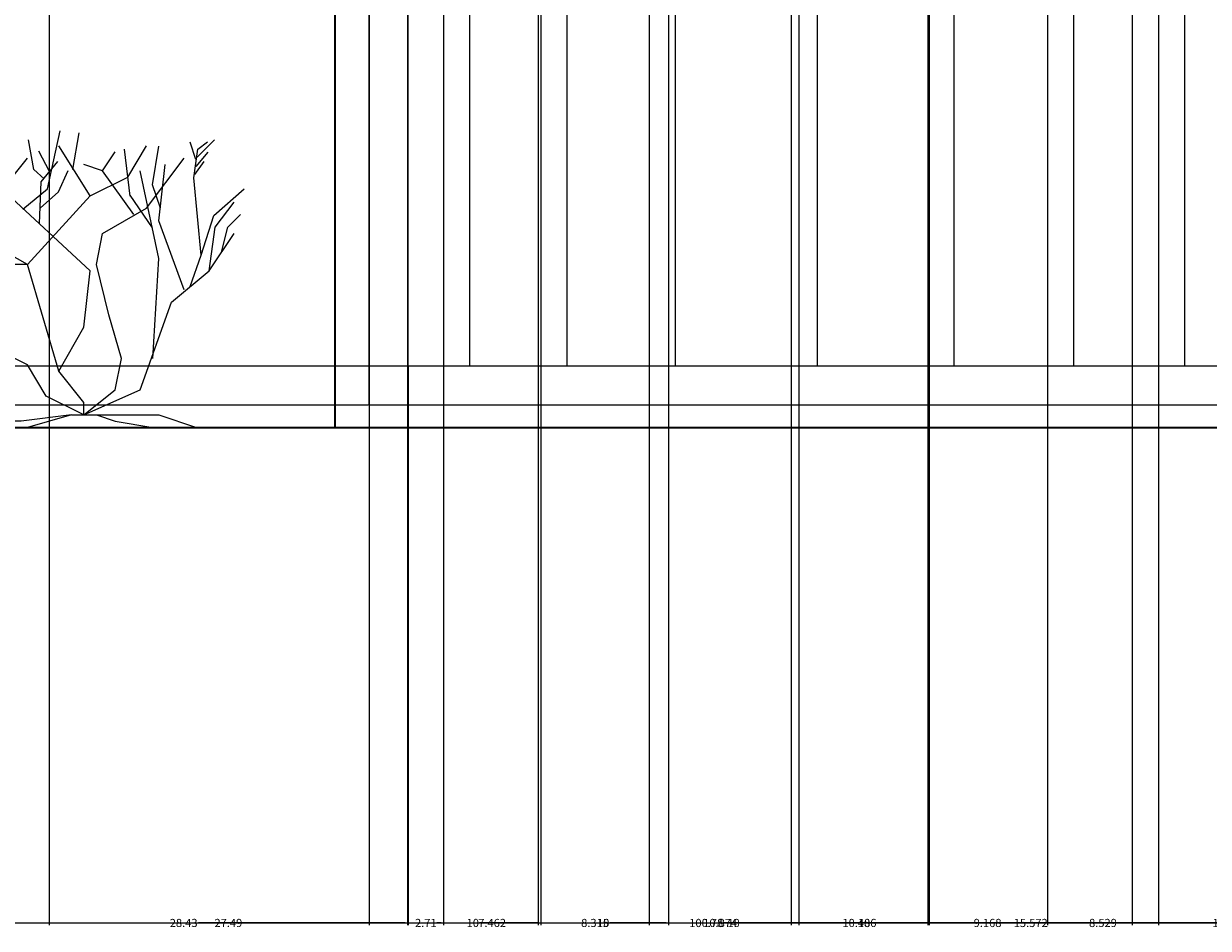
# Model space of a CAD drawing. Units: inches. Extents: x -13 to 809, y 112 to 656.
# Tile 18 of 55: x 339 to 430, y 112 to 181. Entities that reach past the tile are written whole.
import ezdxf

# ---------------------------------------------------------------- set-up
doc = ezdxf.new("R2010")
doc.units = ezdxf.units.IN
doc.header["$MEASUREMENT"] = 0
for name, color, linetype, lineweight in [('A-ANNO-DIMS', 2, 'Continuous', 18), ('A-DOOR', 4, 'Continuous', 25), ('A-ELEV', 7, 'Continuous', 35), ('L-PLNT', 3, 'Continuous', 18)]:
    doc.layers.add(name, color=color, linetype=linetype, lineweight=lineweight)
doc.styles.get("Standard").update_dxf_attribs({"font": 'arial.ttf'})
doc.dimstyles.get("Standard").update_dxf_attribs({"dimtxt": 0.625, "dimasz": 0.18, "dimexe": 0.18, "dimexo": 0.0625, "dimgap": 0.09, "dimtad": 0, "dimtih": 1, "dimtoh": 1, "dimdec": 4, "dimzin": 0, "dimdsep": 46, "dimlunit": 4, "dimtxsty": 'Standard', "dimcen": 0.09, "dimadec": 0, "dimazin": 0, "dimtfac": 1, "dimtdec": 4, "dimtofl": 0, "dimtmove": 0, "dimatfit": 3, "dimfxl": 1, "dimtolj": 1, "dimtzin": 0, "dimarcsym": 0})

# ---------------------------------------------------------------- blocks, each defined once
blk = doc.blocks.new('Shrub - elevation')
for p, q in [((-11.433, 18.289), (-10.457, 22.749)), ((-12.471, 19.775), (-12.898, 22.044)), ((-9.48, 19.775), (-8.992, 22.592)), ((-0.508, 21.888), (-0.081, 20.558)), ((0.041, 20.714), (1.384, 22.044)), ((0.102, 21.34), (0.835, 21.888)), ((-11.28, 19.619), (-12.104, 21.184)), ((-8.16, 17.76), (-10.56, 21.6)), ((-7.2, 19.68), (-6.24, 21.12)), ((-5.086, 17.741), (-5.513, 21.34)), ((-5.28, 19.2), (-3.84, 21.6)), ((-3.377, 18.602), (-2.888, 21.575)), ((-0.203, 19.149), (0.102, 21.34)), ((-0.02, 20.01), (0.896, 21.105)), ((-14.88, 18.24), (-12.96, 20.64)), ((-11.921, 18.836), (-10.64, 20.401)), ((-7.2, 19.68), (-8.64, 20.16)), ((-3.84, 16.8), (-0.96, 20.64)), ((-2.88, 15.84), (-2.4, 20.16)), ((-0.142, 19.384), (0.59, 20.401)), ((-14.88, 18.24), (-17.76, 19.2)), ((-16.8, 16.32), (-15.36, 19.68)), ((-11.677, 19.071), (-12.471, 19.775)), ((-10.579, 18.054), (-9.846, 19.697)), ((-8.16, 17.76), (-5.28, 19.2)), ((-4.8, 16.32), (-7.2, 19.68)), ((-2.88, 12.96), (-4.32, 19.68)), ((0.346, 13.203), (-0.203, 19.149)), ((-16.8, 16.32), (-18.72, 18.72)), ((-8.16, 12), (-14.88, 18.24)), ((-13.325, 16.724), (-11.433, 18.289)), ((-12.043, 15.628), (-11.921, 18.836)), ((-2.766, 16.802), (-3.377, 18.602)), ((1.323, 16.254), (3.642, 18.289)), ((-12.96, 12.48), (-8.16, 17.76)), ((-11.982, 16.802), (-10.579, 18.054)), ((-3.377, 15.315), (-5.086, 17.819)), ((1.44, 15.36), (2.88, 17.28)), ((-18.24, 11.04), (-21.755, 16.655)), ((-7.2, 14.88), (-3.84, 16.8)), ((-12.96, 12.48), (-19.68, 16.32)), ((-16.8, 12.48), (-16.8, 16.32)), ((-0.96, 10.56), (-2.88, 15.84)), ((0.346, 13.203), (1.323, 16.254)), ((2.4, 15.36), (3.36, 16.32)), ((-13.92, 12.48), (-19.2, 14.88)), ((-7.68, 12.48), (-7.2, 14.88)), ((0.96, 12), (1.44, 15.36)), ((0.96, 12), (2.88, 14.88)), ((1.92, 13.44), (2.4, 15.36)), ((-16.8, 12.48), (-17.76, 12.96)), ((-3.36, 5.28), (-2.88, 12.96)), ((-0.48, 10.8), (0.346, 13.203)), ((-17.76, 8.64), (-23.663, 11.961)), ((-15.84, 8.16), (-16.8, 12.48)), ((-12.96, 12.48), (-13.92, 12.48)), ((-10.56, 4.32), (-12.96, 12.48)), ((-8.64, 7.68), (-8.16, 12)), ((-6.72, 8.64), (-7.68, 12.48)), ((-1.92, 9.6), (0.96, 12)), ((-18.24, 11.04), (-20.16, 11.52)), ((-15.84, 8.16), (-18.24, 11.04)), ((-17.76, 8.64), (-23.128, 9.222)), ((-4.32, 2.88), (-1.92, 9.6)), ((-14.88, 5.76), (-17.76, 8.64)), ((-5.76, 5.28), (-6.72, 8.64)), ((-14.88, 5.76), (-15.84, 8.16)), ((-10.56, 4.32), (-8.64, 7.68)), ((-16.32, 7.2), (-18.24, 7.2)), ((-12.96, 4.8), (-14.88, 5.76)), ((-11.52, 2.4), (-12.96, 4.8)), ((-6.24, 2.88), (-5.76, 5.28)), ((-8.64, 1.92), (-10.56, 4.32)), ((-8.64, 0.96), (-4.32, 2.88)), ((-8.64, 0.96), (-6.24, 2.88)), ((-8.64, 0.96), (-11.52, 2.4)), ((-8.64, 0.96), (-8.64, 1.92)), ((-9.6, 0.96), (-13.44, 0.48)), ((-9.6, 0.96), (-12.96, 0)), ((-9.6, 0.96), (-7.68, 0.96)), ((-8.64, 0.96), (-2.88, 0.96)), ((-7.68, 0.96), (-6.24, 0.48)), ((-2.88, 0.96), (0, 0)), ((-15.84, 0.48), (-17.76, 0)), ((-13.44, 0.48), (-15.84, 0.48)), ((-6.24, 0.48), (-3.36, 0))]:
    blk.add_line(p, q)
blk = doc.blocks.new('*D19')
at = {"layer": 'A-ANNO-DIMS', "color": 0, "lineweight": -2, "transparency": 16777216}
for p, q in [((337.507, 306.457), (337.507, 112.34)), ((365.938, 210.722), (365.938, 112.34)), ((337.687, 112.52), (350.573, 112.52)), ((365.758, 112.52), (352.873, 112.52))]:
    blk.add_line(p, q, dxfattribs=at)
at = {"layer": 'A-ANNO-DIMS', "color": 0, "transparency": 16777216}
for points in [[(337.687, 112.55), (337.687, 112.49), (337.507, 112.52)], [(365.758, 112.55), (365.758, 112.49), (365.938, 112.52)]]:
    blk.add_solid(points, dxfattribs=at)
at = {"layer": 'Defpoints', "color": 0, "transparency": 16777216}
for p in [(337.507, 306.52), (365.938, 210.785), (365.938, 112.52)]:
    blk.add_point(p, dxfattribs=at)
at = {"layer": 'A-ANNO-DIMS', "color": 0, "transparency": 16777216, "insert": (351.723, 112.52), "char_height": 0.625, "attachment_point": 5}
blk.add_mtext('\\A1;28.43', dxfattribs=at)
blk = doc.blocks.new('*D20')
at = {"layer": 'A-ANNO-DIMS', "color": 0, "lineweight": -2, "transparency": 16777216}
for p, q in [((365.938, 210.722), (365.938, 112.34)), ((607.574, 209.813), (607.574, 112.34)), ((366.118, 112.52), (485.365, 112.52)), ((607.394, 112.52), (488.148, 112.52))]:
    blk.add_line(p, q, dxfattribs=at)
at = {"layer": 'A-ANNO-DIMS', "color": 0, "transparency": 16777216}
for points in [[(366.118, 112.55), (366.118, 112.49), (365.938, 112.52)], [(607.394, 112.55), (607.394, 112.49), (607.574, 112.52)]]:
    blk.add_solid(points, dxfattribs=at)
at = {"layer": 'Defpoints', "color": 0, "transparency": 16777216}
for p in [(365.938, 210.785), (607.574, 209.875), (607.574, 112.52)]:
    blk.add_point(p, dxfattribs=at)
at = {"layer": 'A-ANNO-DIMS', "color": 0, "transparency": 16777216, "insert": (486.756, 112.52), "char_height": 0.625, "attachment_point": 5}
blk.add_mtext('\\A1;241.64', dxfattribs=at)
blk = doc.blocks.new('*D51')
at = {"layer": 'A-ANNO-DIMS', "color": 0, "lineweight": -2, "transparency": 16777216}
for p, q in [((341.407, 288.388), (341.407, 112.34)), ((442.184, 288.388), (442.184, 112.34)), ((341.587, 112.52), (390.437, 112.52)), ((442.004, 112.52), (393.154, 112.52))]:
    blk.add_line(p, q, dxfattribs=at)
at = {"layer": 'A-ANNO-DIMS', "color": 0, "transparency": 16777216}
for points in [[(341.587, 112.55), (341.587, 112.49), (341.407, 112.52)], [(442.004, 112.55), (442.004, 112.49), (442.184, 112.52)]]:
    blk.add_solid(points, dxfattribs=at)
at = {"layer": 'Defpoints', "color": 0, "transparency": 16777216}
for p in [(341.407, 288.451), (442.184, 288.451), (442.184, 112.52)]:
    blk.add_point(p, dxfattribs=at)
at = {"layer": 'A-ANNO-DIMS', "color": 0, "transparency": 16777216, "insert": (391.796, 112.52), "char_height": 0.625, "attachment_point": 5}
blk.add_mtext('\\A1;100.78', dxfattribs=at)
blk = doc.blocks.new('*D74')
at = {"layer": 'A-ANNO-DIMS', "color": 0, "lineweight": -2, "transparency": 16777216}
for p, q in [((341.407, 210.722), (341.407, 112.34)), ((368.897, 210.711), (368.897, 112.34)), ((341.587, 112.52), (354.001, 112.52)), ((368.717, 112.52), (356.302, 112.52))]:
    blk.add_line(p, q, dxfattribs=at)
at = {"layer": 'A-ANNO-DIMS', "color": 0, "transparency": 16777216}
for points in [[(341.587, 112.55), (341.587, 112.49), (341.407, 112.52)], [(368.717, 112.55), (368.717, 112.49), (368.897, 112.52)]]:
    blk.add_solid(points, dxfattribs=at)
at = {"layer": 'Defpoints', "color": 0, "transparency": 16777216}
for p in [(341.407, 210.785), (368.897, 210.774), (368.897, 112.52)]:
    blk.add_point(p, dxfattribs=at)
at = {"layer": 'A-ANNO-DIMS', "color": 0, "transparency": 16777216, "insert": (355.152, 112.52), "char_height": 0.625, "attachment_point": 5}
blk.add_mtext('\\A1;27.49', dxfattribs=at)
blk = doc.blocks.new('*D75')
at = {"layer": 'A-ANNO-DIMS', "color": 0, "lineweight": -2, "transparency": 16777216}
for p, q in [((378.897, 222.711), (378.897, 112.34)), ((368.897, 216.711), (368.897, 112.34)), ((369.077, 112.52), (373.389, 112.52)), ((378.717, 112.52), (374.404, 112.52))]:
    blk.add_line(p, q, dxfattribs=at)
at = {"layer": 'A-ANNO-DIMS', "color": 0, "transparency": 16777216}
for points in [[(369.077, 112.55), (369.077, 112.49), (368.897, 112.52)], [(378.717, 112.55), (378.717, 112.49), (378.897, 112.52)]]:
    blk.add_solid(points, dxfattribs=at)
at = {"layer": 'Defpoints', "color": 0, "transparency": 16777216}
for p in [(378.897, 222.774), (368.897, 216.774), (378.897, 112.52)]:
    blk.add_point(p, dxfattribs=at)
at = {"layer": 'A-ANNO-DIMS', "color": 0, "transparency": 16777216, "insert": (373.897, 112.52), "char_height": 0.625, "attachment_point": 5}
blk.add_mtext('\\A1;10', dxfattribs=at)
blk = doc.blocks.new('*D76')
at = {"layer": 'A-ANNO-DIMS', "color": 0, "lineweight": -2, "transparency": 16777216}
for p, q in [((388.897, 228.711), (388.897, 112.34)), ((378.897, 222.711), (378.897, 112.34)), ((379.077, 112.52), (383.389, 112.52)), ((388.717, 112.52), (384.404, 112.52))]:
    blk.add_line(p, q, dxfattribs=at)
at = {"layer": 'A-ANNO-DIMS', "color": 0, "transparency": 16777216}
for points in [[(379.077, 112.55), (379.077, 112.49), (378.897, 112.52)], [(388.717, 112.55), (388.717, 112.49), (388.897, 112.52)]]:
    blk.add_solid(points, dxfattribs=at)
at = {"layer": 'Defpoints', "color": 0, "transparency": 16777216}
for p in [(388.897, 228.774), (378.897, 222.774), (388.897, 112.52)]:
    blk.add_point(p, dxfattribs=at)
at = {"layer": 'A-ANNO-DIMS', "color": 0, "transparency": 16777216, "insert": (383.897, 112.52), "char_height": 0.625, "attachment_point": 5}
blk.add_mtext('\\A1;10', dxfattribs=at)
blk = doc.blocks.new('*D77')
at = {"layer": 'A-ANNO-DIMS', "color": 0, "lineweight": -2, "transparency": 16777216}
for p, q in [((398.897, 234.711), (398.897, 112.34)), ((388.897, 228.711), (388.897, 112.34)), ((389.077, 112.52), (393.389, 112.52)), ((398.717, 112.52), (394.404, 112.52))]:
    blk.add_line(p, q, dxfattribs=at)
at = {"layer": 'A-ANNO-DIMS', "color": 0, "transparency": 16777216}
for points in [[(389.077, 112.55), (389.077, 112.49), (388.897, 112.52)], [(398.717, 112.55), (398.717, 112.49), (398.897, 112.52)]]:
    blk.add_solid(points, dxfattribs=at)
at = {"layer": 'Defpoints', "color": 0, "transparency": 16777216}
for p in [(398.897, 234.774), (388.897, 228.774), (398.897, 112.52)]:
    blk.add_point(p, dxfattribs=at)
at = {"layer": 'A-ANNO-DIMS', "color": 0, "transparency": 16777216, "insert": (393.897, 112.52), "char_height": 0.625, "attachment_point": 5}
blk.add_mtext('\\A1;10', dxfattribs=at)
blk = doc.blocks.new('*D78')
at = {"layer": 'A-ANNO-DIMS', "color": 0, "lineweight": -2, "transparency": 16777216}
for p, q in [((408.897, 238.78), (408.897, 112.34)), ((398.897, 234.711), (398.897, 112.34)), ((399.077, 112.52), (403.389, 112.52)), ((408.717, 112.52), (404.404, 112.52))]:
    blk.add_line(p, q, dxfattribs=at)
at = {"layer": 'A-ANNO-DIMS', "color": 0, "transparency": 16777216}
for points in [[(399.077, 112.55), (399.077, 112.49), (398.897, 112.52)], [(408.717, 112.55), (408.717, 112.49), (408.897, 112.52)]]:
    blk.add_solid(points, dxfattribs=at)
at = {"layer": 'Defpoints', "color": 0, "transparency": 16777216}
for p in [(408.897, 238.843), (398.897, 234.774), (408.897, 112.52)]:
    blk.add_point(p, dxfattribs=at)
at = {"layer": 'A-ANNO-DIMS', "color": 0, "transparency": 16777216, "insert": (403.897, 112.52), "char_height": 0.625, "attachment_point": 5}
blk.add_mtext('\\A1;10', dxfattribs=at)
blk = doc.blocks.new('*D79')
at = {"layer": 'A-ANNO-DIMS', "color": 0, "lineweight": -2, "transparency": 16777216}
for p, q in [((408.897, 238.78), (408.897, 112.34)), ((424.469, 238.78), (424.469, 112.34)), ((409.077, 112.52), (415.328, 112.52)), ((424.289, 112.52), (418.037, 112.52))]:
    blk.add_line(p, q, dxfattribs=at)
at = {"layer": 'A-ANNO-DIMS', "color": 0, "transparency": 16777216}
for points in [[(409.077, 112.55), (409.077, 112.49), (408.897, 112.52)], [(424.289, 112.55), (424.289, 112.49), (424.469, 112.52)]]:
    blk.add_solid(points, dxfattribs=at)
at = {"layer": 'Defpoints', "color": 0, "transparency": 16777216}
for p in [(408.897, 238.843), (424.469, 238.843), (424.469, 112.52)]:
    blk.add_point(p, dxfattribs=at)
at = {"layer": 'A-ANNO-DIMS', "color": 0, "transparency": 16777216, "insert": (416.683, 112.52), "char_height": 0.625, "attachment_point": 5}
blk.add_mtext('\\A1;15.572', dxfattribs=at)
blk = doc.blocks.new('*D130')
at = {"layer": 'A-ANNO-DIMS', "color": 0, "lineweight": -2, "transparency": 16777216}
for p, q in [((365.938, 152.152), (365.938, 112.34)), ((608.694, 150.457), (608.694, 112.34)), ((366.118, 112.52), (485.924, 112.52)), ((608.514, 112.52), (488.709, 112.52))]:
    blk.add_line(p, q, dxfattribs=at)
at = {"layer": 'A-ANNO-DIMS', "color": 0, "transparency": 16777216}
for points in [[(366.118, 112.55), (366.118, 112.49), (365.938, 112.52)], [(608.514, 112.55), (608.514, 112.49), (608.694, 112.52)]]:
    blk.add_solid(points, dxfattribs=at)
at = {"layer": 'Defpoints', "color": 0, "transparency": 16777216}
for p in [(365.938, 152.214), (608.694, 150.52), (608.694, 112.52)]:
    blk.add_point(p, dxfattribs=at)
at = {"layer": 'A-ANNO-DIMS', "color": 0, "transparency": 16777216, "insert": (487.316, 112.52), "char_height": 0.625, "attachment_point": 5}
blk.add_mtext('\\A1;242.76', dxfattribs=at)
blk = doc.blocks.new('*D131')
at = {"layer": 'A-ANNO-DIMS', "color": 0, "lineweight": -2, "transparency": 16777216}
for p, q in [((368.876, 155.214), (-12.099, 155.214)), ((-11.919, 155.034), (-11.919, 154.123)), ((-11.919, 152.394), (-11.919, 153.305)), ((365.876, 152.214), (-12.099, 152.214))]:
    blk.add_line(p, q, dxfattribs=at)
at = {"layer": 'A-ANNO-DIMS', "color": 0, "transparency": 16777216}
for points in [[(-11.949, 155.034), (-11.889, 155.034), (-11.919, 155.214)], [(-11.949, 152.394), (-11.889, 152.394), (-11.919, 152.214)]]:
    blk.add_solid(points, dxfattribs=at)
at = {"layer": 'Defpoints', "color": 0, "transparency": 16777216}
for p in [(368.938, 155.214), (-11.919, 152.214), (365.938, 152.214)]:
    blk.add_point(p, dxfattribs=at)
at = {"layer": 'A-ANNO-DIMS', "color": 0, "transparency": 16777216, "insert": (-11.919, 153.714), "char_height": 0.625, "attachment_point": 5}
blk.add_mtext('\\A1;3.00', dxfattribs=at)
blk = doc.blocks.new('*D134')
at = {"layer": 'A-ANNO-DIMS', "color": 0, "lineweight": -2, "transparency": 16777216}
for p, q in [((368.938, 155.152), (368.938, 112.34)), ((371.65, 155.152), (371.65, 112.34)), ((369.118, 112.52), (369.447, 112.52)), ((371.47, 112.52), (371.141, 112.52))]:
    blk.add_line(p, q, dxfattribs=at)
at = {"layer": 'A-ANNO-DIMS', "color": 0, "transparency": 16777216}
for points in [[(369.118, 112.55), (369.118, 112.49), (368.938, 112.52)], [(371.47, 112.55), (371.47, 112.49), (371.65, 112.52)]]:
    blk.add_solid(points, dxfattribs=at)
at = {"layer": 'Defpoints', "color": 0, "transparency": 16777216}
for p in [(368.938, 155.214), (371.65, 155.214), (371.65, 112.52)]:
    blk.add_point(p, dxfattribs=at)
at = {"layer": 'A-ANNO-DIMS', "color": 0, "transparency": 16777216, "insert": (370.294, 112.52), "char_height": 0.625, "attachment_point": 5}
blk.add_mtext('\\A1;2.71', dxfattribs=at)
blk = doc.blocks.new('*D135')
at = {"layer": 'A-ANNO-DIMS', "color": 0, "lineweight": -2, "transparency": 16777216}
for p, q in [((371.65, 155.152), (371.65, 112.34)), ((379.112, 155.152), (379.112, 112.34)), ((371.83, 112.52), (374.242, 112.52)), ((378.932, 112.52), (376.52, 112.52))]:
    blk.add_line(p, q, dxfattribs=at)
at = {"layer": 'A-ANNO-DIMS', "color": 0, "transparency": 16777216}
for points in [[(371.83, 112.55), (371.83, 112.49), (371.65, 112.52)], [(378.932, 112.55), (378.932, 112.49), (379.112, 112.52)]]:
    blk.add_solid(points, dxfattribs=at)
at = {"layer": 'Defpoints', "color": 0, "transparency": 16777216}
for p in [(371.65, 155.214), (379.112, 155.214), (379.112, 112.52)]:
    blk.add_point(p, dxfattribs=at)
at = {"layer": 'A-ANNO-DIMS', "color": 0, "transparency": 16777216, "insert": (375.381, 112.52), "char_height": 0.625, "attachment_point": 5}
blk.add_mtext('\\A1;7.462', dxfattribs=at)
blk = doc.blocks.new('*D136')
at = {"layer": 'A-ANNO-DIMS', "color": 0, "lineweight": -2, "transparency": 16777216}
for p, q in [((379.112, 155.152), (379.112, 112.34)), ((387.428, 155.152), (387.428, 112.34)), ((379.292, 112.52), (382.123, 112.52)), ((387.248, 112.52), (384.417, 112.52))]:
    blk.add_line(p, q, dxfattribs=at)
at = {"layer": 'A-ANNO-DIMS', "color": 0, "transparency": 16777216}
for points in [[(379.292, 112.55), (379.292, 112.49), (379.112, 112.52)], [(387.248, 112.55), (387.248, 112.49), (387.428, 112.52)]]:
    blk.add_solid(points, dxfattribs=at)
at = {"layer": 'Defpoints', "color": 0, "transparency": 16777216}
for p in [(379.112, 155.214), (387.428, 155.214), (387.428, 112.52)]:
    blk.add_point(p, dxfattribs=at)
at = {"layer": 'A-ANNO-DIMS', "color": 0, "transparency": 16777216, "insert": (383.27, 112.52), "char_height": 0.625, "attachment_point": 5}
blk.add_mtext('\\A1;8.315', dxfattribs=at)
blk = doc.blocks.new('*D137')
at = {"layer": 'A-ANNO-DIMS', "color": 0, "lineweight": -2, "transparency": 16777216}
for p, q in [((387.428, 155.152), (387.428, 112.34)), ((398.301, 155.152), (398.301, 112.34)), ((387.608, 112.52), (391.508, 112.52)), ((398.121, 112.52), (394.221, 112.52))]:
    blk.add_line(p, q, dxfattribs=at)
at = {"layer": 'A-ANNO-DIMS', "color": 0, "transparency": 16777216}
for points in [[(387.608, 112.55), (387.608, 112.49), (387.428, 112.52)], [(398.121, 112.55), (398.121, 112.49), (398.301, 112.52)]]:
    blk.add_solid(points, dxfattribs=at)
at = {"layer": 'Defpoints', "color": 0, "transparency": 16777216}
for p in [(387.428, 155.214), (398.301, 155.214), (398.301, 112.52)]:
    blk.add_point(p, dxfattribs=at)
at = {"layer": 'A-ANNO-DIMS', "color": 0, "transparency": 16777216, "insert": (392.865, 112.52), "char_height": 0.625, "attachment_point": 5}
blk.add_mtext('\\A1;10.874', dxfattribs=at)
blk = doc.blocks.new('*D138')
at = {"layer": 'A-ANNO-DIMS', "color": 0, "lineweight": -2, "transparency": 16777216}
for p, q in [((398.301, 155.152), (398.301, 112.34)), ((408.787, 155.152), (408.787, 112.34)), ((398.481, 112.52), (402.187, 112.52)), ((408.607, 112.52), (404.902, 112.52))]:
    blk.add_line(p, q, dxfattribs=at)
at = {"layer": 'A-ANNO-DIMS', "color": 0, "transparency": 16777216}
for points in [[(398.481, 112.55), (398.481, 112.49), (398.301, 112.52)], [(408.607, 112.55), (408.607, 112.49), (408.787, 112.52)]]:
    blk.add_solid(points, dxfattribs=at)
at = {"layer": 'Defpoints', "color": 0, "transparency": 16777216}
for p in [(398.301, 155.214), (408.787, 155.214), (408.787, 112.52)]:
    blk.add_point(p, dxfattribs=at)
at = {"layer": 'A-ANNO-DIMS', "color": 0, "transparency": 16777216, "insert": (403.544, 112.52), "char_height": 0.625, "attachment_point": 5}
blk.add_mtext('\\A1;10.486', dxfattribs=at)
blk = doc.blocks.new('*D139')
at = {"layer": 'A-ANNO-DIMS', "color": 0, "lineweight": -2, "transparency": 16777216}
for p, q in [((408.787, 155.152), (408.787, 112.34)), ((417.955, 155.152), (417.955, 112.34)), ((408.967, 112.52), (412.226, 112.52)), ((417.775, 112.52), (414.517, 112.52))]:
    blk.add_line(p, q, dxfattribs=at)
at = {"layer": 'A-ANNO-DIMS', "color": 0, "transparency": 16777216}
for points in [[(408.967, 112.55), (408.967, 112.49), (408.787, 112.52)], [(417.775, 112.55), (417.775, 112.49), (417.955, 112.52)]]:
    blk.add_solid(points, dxfattribs=at)
at = {"layer": 'Defpoints', "color": 0, "transparency": 16777216}
for p in [(408.787, 155.214), (417.955, 155.214), (417.955, 112.52)]:
    blk.add_point(p, dxfattribs=at)
at = {"layer": 'A-ANNO-DIMS', "color": 0, "transparency": 16777216, "insert": (413.371, 112.52), "char_height": 0.625, "attachment_point": 5}
blk.add_mtext('\\A1;9.168', dxfattribs=at)
blk = doc.blocks.new('*D140')
at = {"layer": 'A-ANNO-DIMS', "color": 0, "lineweight": -2, "transparency": 16777216}
for p, q in [((417.955, 155.152), (417.955, 112.34)), ((426.484, 155.152), (426.484, 112.34)), ((418.135, 112.52), (421.074, 112.52)), ((426.304, 112.52), (423.365, 112.52))]:
    blk.add_line(p, q, dxfattribs=at)
at = {"layer": 'A-ANNO-DIMS', "color": 0, "transparency": 16777216}
for points in [[(418.135, 112.55), (418.135, 112.49), (417.955, 112.52)], [(426.304, 112.55), (426.304, 112.49), (426.484, 112.52)]]:
    blk.add_solid(points, dxfattribs=at)
at = {"layer": 'Defpoints', "color": 0, "transparency": 16777216}
for p in [(417.955, 155.214), (426.484, 155.214), (426.484, 112.52)]:
    blk.add_point(p, dxfattribs=at)
at = {"layer": 'A-ANNO-DIMS', "color": 0, "transparency": 16777216, "insert": (422.22, 112.52), "char_height": 0.625, "attachment_point": 5}
blk.add_mtext('\\A1;8.529', dxfattribs=at)
blk = doc.blocks.new('*D141')
at = {"layer": 'A-ANNO-DIMS', "color": 0, "lineweight": -2, "transparency": 16777216}
for p, q in [((426.484, 155.152), (426.484, 112.34)), ((437.358, 155.152), (437.358, 112.34)), ((426.664, 112.52), (430.564, 112.52)), ((437.178, 112.52), (433.278, 112.52))]:
    blk.add_line(p, q, dxfattribs=at)
at = {"layer": 'A-ANNO-DIMS', "color": 0, "transparency": 16777216}
for points in [[(426.664, 112.55), (426.664, 112.49), (426.484, 112.52)], [(437.178, 112.55), (437.178, 112.49), (437.358, 112.52)]]:
    blk.add_solid(points, dxfattribs=at)
at = {"layer": 'Defpoints', "color": 0, "transparency": 16777216}
for p in [(426.484, 155.214), (437.358, 155.214), (437.358, 112.52)]:
    blk.add_point(p, dxfattribs=at)
at = {"layer": 'A-ANNO-DIMS', "color": 0, "transparency": 16777216, "insert": (431.921, 112.52), "char_height": 0.625, "attachment_point": 5}
blk.add_mtext('\\A1;10.874', dxfattribs=at)

msp = doc.modelspace()

# ---------------------------------------------------------------- linework, layer by layer
at = {"layer": 'A-DOOR'}
for p, q in [((371.6498, 207.3724), (371.6498, 155.2141)), ((373.6498, 207.3724), (373.6498, 155.2141)), ((379.1123, 207.3724), (379.1123, 155.2141)), ((381.1123, 207.3724), (381.1123, 155.2141)), ((387.4276, 207.3724), (387.4276, 155.2141)), ((389.4276, 207.3724), (389.4276, 155.2141)), ((398.3015, 207.3724), (398.3015, 155.2141)), ((400.3015, 207.3724), (400.3015, 155.2141)), ((408.7873, 207.3724), (408.7873, 155.2141)), ((410.7873, 207.3724), (410.7873, 155.2141)), ((417.9555, 207.3724), (417.9555, 155.2141)), ((419.9555, 207.3724), (419.9555, 155.2141)), ((426.484, 207.3724), (426.484, 155.2141)), ((428.484, 207.3724), (428.484, 155.2141))]:
    msp.add_line(p, q, dxfattribs=at)
for points in [[(365.9383, 210.7849), (607.5741, 209.8753), (607.5741, 152.2141), (365.9383, 152.2141)], [(368.9383, 207.7736), (604.5741, 206.8866), (604.5741, 155.2141), (368.9383, 155.2141)]]:
    msp.add_lwpolyline(points, close=True, dxfattribs=at)
at = {"layer": 'A-ELEV'}
for p, q in [((363.3158, 210.7849), (363.3158, 150.5199)), ((109.5888, 150.5199), (649.5888, 150.5199))]:
    msp.add_line(p, q, dxfattribs=at)

# ---------------------------------------------------------------- block references
at = {"layer": 'L-PLNT'}
msp.add_blockref('Shrub - elevation', (352.7114, 150.5199), dxfattribs=at)

# ---------------------------------------------------------------- dimensions: what is measured, and where the dimension line sits
at = {"layer": 'A-ANNO-DIMS'}
for base, p1, p2, override, picture, middle in [((365.9383, 112.5199), (337.5074, 306.5199), (365.9383, 210.7849), {"dimdec": 2, "dimlfac": 1, "dimrnd": 0, "dimzin": 0, "dimdsep": 46, "dimlunit": 2}, '*D19', (351.7228, 112.5199)), ((442.1845, 112.5199), (341.4072, 288.4508), (442.1845, 288.4508), {"dimdec": 2, "dimlfac": 1, "dimrnd": 0, "dimzin": 0, "dimdsep": 46, "dimlunit": 2}, '*D51', (391.7958, 112.5199)), ((408.8966, 112.5199), (398.8966, 234.7738), (408.8966, 238.8429), {"dimdec": 0, "dimlfac": 1, "dimrnd": 0, "dimzin": 0, "dimdsep": 46, "dimlunit": 2}, '*D78', (403.8966, 112.5199)), ((424.469, 112.5199), (408.8966, 238.8429), (424.469, 238.8429), {"dimdec": 3, "dimlfac": 1, "dimrnd": 0, "dimzin": 0, "dimdsep": 46, "dimlunit": 2}, '*D79', (416.6828, 112.5199)), ((398.8966, 112.5199), (388.8966, 228.7738), (398.8966, 234.7738), {"dimdec": 0, "dimlfac": 1, "dimrnd": 0, "dimzin": 0, "dimdsep": 46, "dimlunit": 2}, '*D77', (393.8966, 112.5199)), ((388.8966, 112.5199), (378.8966, 222.7738), (388.8966, 228.7738), {"dimdec": 0, "dimlfac": 1, "dimrnd": 0, "dimzin": 0, "dimdsep": 46, "dimlunit": 2}, '*D76', (383.8966, 112.5199)), ((378.8966, 112.5199), (368.8966, 216.7738), (378.8966, 222.7738), {"dimdec": 0, "dimlfac": 1, "dimrnd": 0, "dimzin": 0, "dimdsep": 46, "dimlunit": 2}, '*D75', (373.8966, 112.5199)), ((368.8966, 112.5199), (341.4072, 210.7849), (368.8966, 210.7738), {"dimdec": 2, "dimlfac": 1, "dimrnd": 0, "dimzin": 0, "dimdsep": 46, "dimlunit": 2}, '*D74', (355.1519, 112.5199)), ((607.5741, 112.5199), (365.9383, 210.7849), (607.5741, 209.8753), {"dimdec": 2, "dimlfac": 1, "dimrnd": 0, "dimzin": 0, "dimdsep": 46, "dimlunit": 2}, '*D20', (486.7562, 112.5199)), ((371.6498, 112.5199), (368.9383, 155.2141), (371.6498, 155.2141), {"dimdec": 2, "dimlfac": 1, "dimrnd": 0, "dimzin": 0, "dimdsep": 46, "dimlunit": 2}, '*D134', (370.294, 112.5199)), ((379.11227, 112.51989), (371.64981, 155.21411), (379.11227, 155.21411), {"dimdec": 3, "dimlfac": 1, "dimrnd": 0, "dimzin": 0, "dimdsep": 46, "dimlunit": 2}, '*D135', (375.38104, 112.51989)), ((387.4276, 112.5199), (379.1123, 155.2141), (387.4276, 155.2141), {"dimdec": 3, "dimlfac": 1, "dimrnd": 0, "dimzin": 0, "dimdsep": 46, "dimlunit": 2}, '*D136', (383.2699, 112.5199)), ((398.3015, 112.5199), (387.4276, 155.2141), (398.3015, 155.2141), {"dimdec": 3, "dimlfac": 1, "dimrnd": 0, "dimzin": 0, "dimdsep": 46, "dimlunit": 2}, '*D137', (392.8645, 112.5199)), ((408.7873, 112.5199), (398.3015, 155.2141), (408.7873, 155.2141), {"dimdec": 3, "dimlfac": 1, "dimrnd": 0, "dimzin": 0, "dimdsep": 46, "dimlunit": 2}, '*D138', (403.5444, 112.5199)), ((417.9555, 112.5199), (408.7873, 155.2141), (417.9555, 155.2141), {"dimdec": 3, "dimlfac": 1, "dimrnd": 0, "dimzin": 0, "dimdsep": 46, "dimlunit": 2}, '*D139', (413.3714, 112.5199)), ((426.484, 112.51989), (417.95547, 155.21411), (426.484, 155.21411), {"dimdec": 3, "dimlfac": 1, "dimrnd": 0, "dimzin": 0, "dimdsep": 46, "dimlunit": 2}, '*D140', (422.21973, 112.51989)), ((437.3579, 112.5199), (426.484, 155.2141), (437.3579, 155.2141), {"dimdec": 3, "dimlfac": 1, "dimrnd": 0, "dimzin": 0, "dimdsep": 46, "dimlunit": 2}, '*D141', (431.9209, 112.5199)), ((608.694, 112.5199), (365.9383, 152.2141), (608.694, 150.5199), {"dimdec": 2, "dimlfac": 1, "dimrnd": 0, "dimzin": 0, "dimdsep": 46, "dimlunit": 2}, '*D130', (487.3161, 112.5199))]:
    dim = msp.add_linear_dim(base=base, p1=p1, p2=p2, dimstyle='Standard', override=override, dxfattribs=at)
    dim.commit()
    dim.dimension.update_dxf_attribs({"geometry": picture, "text_midpoint": middle})
dim = msp.add_linear_dim(base=(-11.9191, 152.2141), p1=(368.9383, 155.2141), p2=(365.9383, 152.2141), angle=90, dimstyle='Standard', override={"dimdec": 2, "dimlfac": 1, "dimrnd": 0, "dimzin": 0, "dimdsep": 46, "dimlunit": 2}, dxfattribs=at)
dim.commit()
dim.dimension.update_dxf_attribs({"geometry": '*D131', "text_midpoint": (-11.9191, 153.7141)})

doc.saveas('drawing.dxf')
